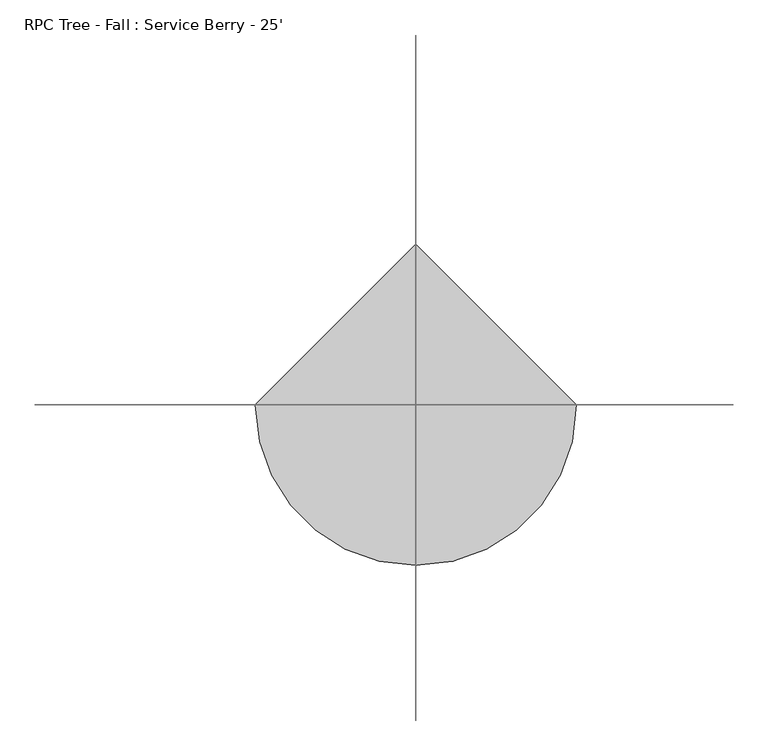
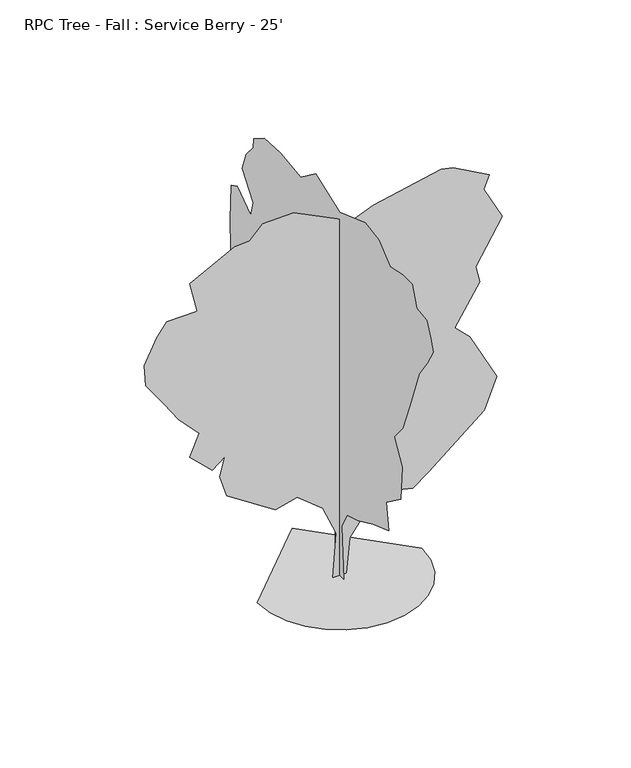
"""IFC4 building model written with IfcOpenShell, lengths in millimetres: geographic element geometry, RPC Tree - Fall : Service Berry - 25'."""

from ifc_helpers import new_model, si_unit, origin, place, context, project, spatial, triangles, source, transform, mapped, element, save


def rpc_tree_fall_service_berry_25_c2e4521a(model_context):
    return source(origin(), model_context, "Body", "Tessellation", [
        triangles([(-439.377505, 0.0, 0.0258158), (-427.7614626, -100.6759497, 0.0258158), (-394.6800516, -193.1311439, 0.0258158), (-342.7816933, -274.7163712, 0.0258158), (-274.7163712, -342.7816933, 0.0258158), (-193.1311439, -394.6800516, 0.0258158), (-100.6759497, -427.7614626, 0.0258158), (1.92e-05, -439.377505, 0.0258158), (100.6759497, -427.7614626, 0.0258158), (193.1311439, -394.6800516, 0.0258158), (274.7163712, -342.7816933, 0.0258158), (342.78242, -274.7163712, 0.0258158), (394.6800516, -193.1311439, 0.0258158), (427.7614626, -100.6759497, 0.0258158), (439.377505, 3.84e-05, 0.0258158), (-5.76e-05, 439.377505, 0.0258158), (-4.7e-06, -39.6248933, 0.0412325), (3.21e-05, -19.527896, 289.0164612), (3.72e-05, -71.7877466, 384.1372358), (2.87e-05, -172.2994031, 412.8547417), (1.97e-05, -312.2968534, 477.4693296), (9e-06, -452.2943038, 527.7248013), (2.91e-05, -430.7563379, 674.901828), (2.48e-05, -563.574212, 771.8219296), (4.58e-05, -577.9333282, 962.0748516), (6.08e-05, -531.2672813, 1041.0464121), (6.98e-05, -502.5497755, 1087.7152931), (7.15e-05, -585.1129045, 1184.6375748), (8.34e-05, -646.1373774, 1346.1721916), (0.0001012, -734.5479692, 1583.5492722), (0.0001048, -807.6734476, 1687.1923645), (0.0001096, -865.1099127, 1784.1145008), (0.0001202, -839.9832487, 1848.7269814), (0.0001339, -804.0819517, 1927.6986145), (0.0001464, -714.3428072, 1942.0576218), (0.0001643, -671.264768, 2049.7474148), (0.0001749, -582.2801923, 2049.8469727), (0.0001859, -465.6271382, 2024.7487953), (0.0002091, -359.1855248, 2113.0939842), (0.0002262, -236.2874305, 2133.5978199), (0.0002443, -0.1649008, 2049.4061565), (0.0002805, 220.9774457, 2132.3746387), (0.0002849, 359.5489474, 2030.395689), (0.0003102, 549.2271953, 2053.339056), (0.0003269, 696.4042219, 2046.1630405), (0.0003312, 796.9130579, 1981.5434383), (0.0003255, 800.6112333, 1929.6117245), (0.0003239, 865.1170343, 1852.3184772), (0.0003162, 901.018404, 1751.8046997), (0.0002884, 797.389555, 1621.697961), (0.0002812, 824.905826, 1533.7794903), (0.0003062, 945.7243961, 1622.9141659), (0.0003098, 1005.1166285, 1593.8615788), (0.0002871, 1012.2997656, 1396.4255196), (0.0002476, 1003.0185734, 1074.1527489), (0.0002152, 865.1170343, 940.5397562), (0.0001746, 735.8921459, 728.7445444), (0.0001458, 571.3945922, 651.790666), (0.000119, 400.8219732, 597.2530792), (0.0001145, 324.6930445, 635.4152847), (9.93e-05, 265.6421794, 567.2113083), (9.37e-05, 290.7702786, 495.417144), (8.52e-05, 272.8217375, 441.5722475), (6.12e-05, 168.5471249, 344.6507289), (5.87e-05, 88.1567102, 404.0842378), (4.13e-05, 40.216327, 305.8619265), (4.3e-06, 35.8446576, 0.0244626), (-36.7229174, 1.6e-06, 3.1e-06), (-18.8427986, -2.84e-05, 245.1134179), (-90.2255883, -4.51e-05, 411.3925126), (-227.6740936, -5.21e-05, 520.799134), (-344.2261545, -4.34e-05, 490.3242499), (-603.749158, -5.23e-05, 660.5014715), (-641.3090384, -6.52e-05, 781.8142702), (-614.5181591, -7.88e-05, 886.6521297), (-680.4320864, -6.96e-05, 833.3548742), (-801.1802393, -7.79e-05, 947.6730417), (-750.7206013, -9.42e-05, 1065.3551754), (-858.6167044, -0.0001033, 1181.0033489), (-937.5882648, -0.0001135, 1295.8762791), (-1034.5104738, -0.0001255, 1432.2842319), (-1042.9880087, -0.0001391, 1549.3689457), (-977.6074064, -0.0001582, 1685.5280766), (-923.2291122, -0.0001689, 1755.353611), (-760.2364449, -0.0001763, 1758.0989376), (-801.1802393, -0.0001948, 1927.6630062), (-560.6725359, -0.0002203, 2053.2963261), (-479.9642355, -0.0002244, 2058.1681217), (-409.9061208, -0.0002358, 2128.6834396), (-246.2428003, -0.0002435, 2133.1285172), (65.4940583, -0.000239, 1980.4837646), (178.801895, -0.0002496, 2028.1696621), (541.3599066, -0.0002744, 2103.5567757), (605.9744946, -0.0002755, 2089.1976231), (798.7479023, -0.0002712, 1982.1906372), (770.1577143, -0.0002615, 1911.0138771), (868.2392275, -0.0002434, 1723.2500473), (727.1657164, -0.0002092, 1487.9995811), (747.1291054, -0.0001991, 1396.3473267), (614.0593935, -0.000168, 1184.3245852), (695.5579073, -0.0001619, 1103.3687708), (838.6959726, -0.0001357, 830.5456707), (772.8602383, -0.0001128, 662.7410151), (473.1558938, -7.03e-05, 416.4029263), (388.7365554, -5.95e-05, 356.6671466), (232.6475182, -5.72e-05, 394.8649604), (150.0481178, -4.52e-05, 323.9064646), (54.2903226, -2.56e-05, 194.9902237), (34.012536, -1.5e-06, 0.0)], [[15, 16, 1], [14, 15, 1], [14, 1, 2], [13, 14, 2], [13, 2, 3], [13, 3, 4], [12, 13, 4], [11, 12, 4], [11, 4, 5], [11, 5, 6], [11, 6, 7], [11, 7, 8], [11, 8, 9], [11, 9, 10], [67, 17, 18], [66, 67, 18], [63, 64, 65], [21, 22, 23], [66, 18, 19], [65, 66, 19], [35, 36, 37], [51, 52, 53], [51, 53, 54], [62, 63, 65], [61, 62, 65], [48, 49, 50], [41, 42, 43], [33, 34, 35], [47, 48, 50], [51, 54, 55], [51, 55, 56], [45, 46, 47], [31, 32, 33], [31, 33, 35], [30, 31, 35], [35, 37, 38], [30, 35, 38], [29, 30, 38], [23, 24, 25], [23, 25, 26], [23, 26, 27], [44, 45, 47], [44, 47, 50], [43, 44, 50], [58, 59, 60], [41, 43, 50], [41, 50, 51], [41, 51, 56], [41, 56, 57], [41, 57, 58], [41, 58, 60], [40, 41, 60], [39, 40, 60], [38, 39, 60], [29, 38, 60], [28, 29, 60], [27, 28, 60], [23, 27, 60], [23, 60, 61], [21, 23, 61], [20, 21, 61], [20, 61, 65], [20, 65, 19], [109, 68, 69], [108, 109, 69], [107, 108, 69], [107, 69, 70], [94, 95, 96], [75, 76, 77], [75, 77, 78], [85, 86, 87], [106, 107, 70], [96, 97, 98], [85, 87, 88], [83, 84, 85], [101, 102, 103], [101, 103, 104], [100, 101, 104], [104, 105, 106], [100, 104, 106], [100, 106, 70], [100, 70, 71], [94, 96, 98], [93, 94, 98], [92, 93, 98], [91, 92, 98], [71, 72, 73], [100, 71, 73], [100, 73, 74], [100, 74, 75], [100, 75, 78], [99, 100, 78], [98, 99, 78], [91, 98, 78], [90, 91, 78], [89, 90, 78], [88, 89, 78], [85, 88, 78], [85, 78, 79], [85, 79, 80], [83, 85, 80], [83, 80, 81], [82, 83, 81]], closed=False),
    ])


if __name__ == "__main__":
    model = new_model("IFC4")
    model_context = context("Model", 3, world=origin())
    ifc_project = project(units=[si_unit("LENGTHUNIT", "METRE", prefix="MILLI")], contexts=[model_context])
    site = spatial("IfcSite", under=ifc_project)
    building = spatial("IfcBuilding", under=site)
    placement = place(None, origin())
    rpc_tree_fall_service_berry_25_shape = rpc_tree_fall_service_berry_25_c2e4521a(model_context)
    element("IfcGeographicElement", 1, ObjectType="RPC Tree - Fall : Service Berry - 25'", at=placement, inside=building, context=model_context, shape_type="MappedRepresentation", body=[
        mapped(rpc_tree_fall_service_berry_25_shape, transform((0.0, 0.0, 0.0), x_axis=(1.0, 0.0, 0.0), y_axis=(0.0, 1.0, 0.0), z_axis=(0.0, 0.0, 1.0))),
    ])
    save(model, "model.ifc")

# Revit data of these elements
# Type "RPC Tree - Fall : Service Berry - 25'"
#   built-in parameter 1005198 = "{2, 15},{39, RPC-16-FVGU-8VG0-7PL0-4000-ST1L-LVER-AU},{1, 0},{1, 0},{2, 13},{1, 8},{5, Color},{1, 0},{1, 0},{3, 0.8},{3, 0.8},{3, 0.8},{1, 8},{7, BBoxMin},{1, 0},{1, 0},{1, 0},{1, 0},{1, 0},{1, 8},{7, BBoxMax},{1, 0},{1, 0},{1, 0},{1, 0},{1, 0},{2, 11},{9, RPCTypeId},{1, 0},{1, 0},{39, RPC-16-FVGU-8VG0-7PL0-4000-ST1L-LVER-AU},{1, 6},{14, RPCPlantHeight},{1, 0},{1, 0},{2, 25},{2, 11},{7, keyword},{1, 0},{1, 0},{39, :RPCs:Fall Trees [General]:Geometry:RPC},{2, 11},{8, category},{1, 0},{1, 0},{20, Fall Trees [General]},{2, 11},{12, LocalizedUID},{1, 0},{1, 0},{20, Service Berry [Fall]},{2, 14},{6, Height},{1, 0},{1, 0},{2, 25},{1, 2},{16, Cast Reflections},{1, 0},{1, 0},{1, 0},{1, 2},{12, Cast Shadows},{1, 0},{1, 0},{1, 1},{1, 2},{9, Lock View},{1, 0},{1, 0},{1, 0},{1, 4},{5, ViewC},{1, 0},{1, 0},{1, 0},{21, assetlibrary_base.fbx},{1, 5},"
#   built-in parameter 1005195 = "RPC-16-FVGU-8VG0-7PL0-4000-ST1L-LVER-AU"
#   Type Comments = "Service Berry"
#   Assembly Code = "G2050500"
#   Height = 7' - 0"
#   Default Elevation = 0
